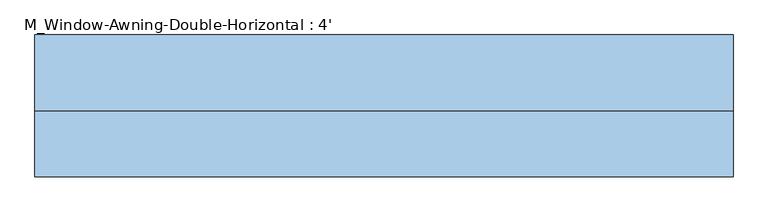
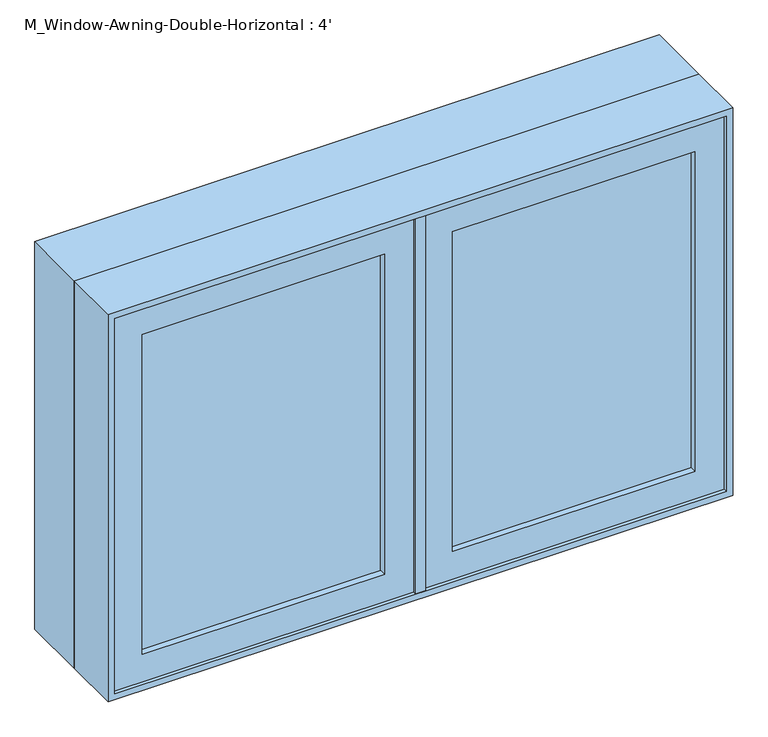
"""IFC4 building model written with IfcOpenShell, lengths in millimetres: window geometry, M_Window-Awning-Double-Horizontal : 4'."""

from ifc_helpers import new_model, si_unit, frame, origin, place, context, project, spatial, polyline, outline, extrude, faceted_brep, source, transform, mapped, element, save


def m_window_awning_double_horizontal_4_e2f7b2f6(model_context):
    return source(origin(), model_context, "Body", "SolidModel", [
        faceted_brep([(577.85, -82.55, 1668.25), (-577.85, -82.55, 1668.25), (-577.85, -19.05, 1668.25), (577.85, -19.05, 1668.25), (596.9, -133.35, 1687.3), (-596.9, -133.35, 1687.3), (-596.9, -82.55, 1687.3), (596.9, -82.55, 1687.3), (609.6, -19.05, 1700.0), (-609.6, -19.05, 1700.0), (-609.6, -133.35, 1700.0), (609.6, -133.35, 1700.0), (-577.85, -82.55, 931.75), (-577.85, -19.05, 931.75), (-596.9, -133.35, 912.7), (-596.9, -82.55, 912.7), (-609.6, -19.05, 900.0), (-609.6, -133.35, 900.0), (577.85, -82.55, 931.75), (577.85, -19.05, 931.75), (596.9, -133.35, 912.7), (596.9, -82.55, 912.7), (609.6, -19.05, 900.0), (609.6, -133.35, 900.0)], [[[0, 1, 2, 3]], [[4, 5, 6, 7]], [[8, 9, 10, 11]], [[1, 12, 13, 2]], [[5, 14, 15, 6]], [[9, 16, 17, 10]], [[12, 18, 19, 13]], [[14, 20, 21, 15]], [[16, 22, 23, 17]], [[9, 8, 22, 16], [3, 2, 13, 19]], [[18, 0, 3, 19]], [[7, 6, 15, 21], [1, 0, 18, 12]], [[20, 4, 7, 21]], [[22, 8, 11, 23]], [[11, 10, 17, 23], [5, 4, 20, 14]]]),
        extrude(outline(polyline([(1700.0, -609.6), (900.0, -609.6), (900.0, 609.6), (1700.0, 609.6), (1700.0, -609.6)]), holes=[polyline([(1680.95, 590.55), (919.05, 590.55), (919.05, -590.55), (1680.95, -590.55), (1680.95, 590.55)])]), frame((0.0, -19.05, 0.0), z_axis=(0.0, 1.0, 0.0), x_axis=(0.0, 0.0, 1.0)), (0.0, 0.0, 1.0), 133.35),
        extrude(outline(polyline([(912.7, 9.525), (912.7, 596.9), (1687.3, 596.9), (1687.3, 9.525), (912.7, 9.525)]), holes=[polyline([(969.85, 539.75), (969.85, 66.675), (1630.15, 66.675), (1630.15, 539.75), (969.85, 539.75)])]), frame((0.0, -127.0, 0.0), z_axis=(0.0, 1.0, 0.0), x_axis=(0.0, 0.0, 1.0)), (0.0, 0.0, 1.0), 44.45),
        extrude(outline(polyline([(1687.3, -9.525), (1687.3, -596.9), (912.7, -596.9), (912.7, -9.525), (1687.3, -9.525)]), holes=[polyline([(1630.15, -539.75), (1630.15, -66.675), (969.85, -66.675), (969.85, -539.75), (1630.15, -539.75)])]), frame((0.0, -127.0, 0.0), z_axis=(0.0, 1.0, 0.0), x_axis=(0.0, 0.0, 1.0)), (0.0, 0.0, 1.0), 44.45),
        extrude(outline(polyline([(539.75, -114.3), (66.675, -114.3), (66.675, -107.95), (539.75, -107.95), (539.75, -114.3)])), frame((0.0, 0.0, 969.85), z_axis=(0.0, 0.0, 1.0), x_axis=(1.0, 0.0, 0.0)), (0.0, 0.0, 1.0), 660.3),
        extrude(outline(polyline([(66.675, -95.25), (539.75, -95.25), (539.75, -101.6), (66.675, -101.6), (66.675, -95.25)])), frame((0.0, 0.0, 969.85), z_axis=(0.0, 0.0, 1.0), x_axis=(1.0, 0.0, 0.0)), (0.0, 0.0, 1.0), 660.3),
        extrude(outline(polyline([(-66.675, -114.3), (-539.75, -114.3), (-539.75, -107.95), (-66.675, -107.95), (-66.675, -114.3)])), frame((0.0, 0.0, 969.85), z_axis=(0.0, 0.0, 1.0), x_axis=(1.0, 0.0, 0.0)), (0.0, 0.0, 1.0), 660.3),
        extrude(outline(polyline([(-539.75, -95.25), (-66.675, -95.25), (-66.675, -101.6), (-539.75, -101.6), (-539.75, -95.25)])), frame((0.0, 0.0, 969.85), z_axis=(0.0, 0.0, 1.0), x_axis=(1.0, 0.0, 0.0)), (0.0, 0.0, 1.0), 660.3),
        faceted_brep([(9.525, -133.35, 1687.3), (9.525, -82.55, 1687.3), (-9.525, -82.55, 1687.3), (-9.525, -133.35, 1687.3), (9.525, -133.35, 912.7), (-9.525, -133.35, 912.7), (-9.525, -82.55, 912.7), (9.525, -82.55, 912.7), (-9.525, -82.55, 1668.25), (-9.525, -82.55, 931.75), (-30.1625, -82.55, 1668.25), (-30.1625, -82.55, 931.75), (-30.1625, -19.05, 1668.25), (-30.1625, -19.05, 931.75), (30.1625, -19.05, 1668.25), (30.1625, -19.05, 931.75), (30.1625, -82.55, 1668.25), (30.1625, -82.55, 931.75), (9.525, -82.55, 1668.25), (9.525, -82.55, 931.75)], [[[0, 1, 2, 3]], [[4, 5, 6, 7]], [[3, 5, 4, 0]], [[2, 8, 9, 6, 5, 3]], [[8, 10, 11, 9]], [[10, 12, 13, 11]], [[12, 14, 15, 13]], [[14, 16, 17, 15]], [[16, 18, 19, 17]], [[0, 4, 7, 19, 18, 1]], [[8, 2, 1, 18]], [[19, 7, 6, 9]], [[9, 11, 13, 15, 17, 19]], [[18, 16, 14, 12, 10, 8]]]),
    ])


if __name__ == "__main__":
    model = new_model("IFC4")
    model_context = context("Model", 3, world=origin())
    ifc_project = project(units=[si_unit("LENGTHUNIT", "METRE", prefix="MILLI")], contexts=[model_context])
    site = spatial("IfcSite", under=ifc_project)
    building = spatial("IfcBuilding", under=site)
    placement = place(None, origin())
    m_window_awning_double_horizontal_4_shape = m_window_awning_double_horizontal_4_e2f7b2f6(model_context)
    element("IfcWindow", 1, ObjectType="M_Window-Awning-Double-Horizontal : 4'", at=placement, inside=building, context=model_context, shape_type="MappedRepresentation", body=[
        mapped(m_window_awning_double_horizontal_4_shape, transform((0.0, 0.0, 0.0), x_axis=(1.0, 0.0, 0.0), y_axis=(0.0, 1.0, 0.0), z_axis=(0.0, 0.0, 1.0))),
    ])
    save(model, "model.ifc")

# Revit data of these elements
# Type "M_Window-Awning-Double-Horizontal : 4'"
#   Type Mark = "28"
#   Fire Rating = "0.5h"
#   Assembly Code = "B2020100"
#   Analytic Construction = "Double glazing - domestic"
#   Window Inset [instance default] = 0' - 0"
#   Wall Thickness [instance default] = 0' - 5.90551"
#   Interior Wall Closure [instance default] = 0' - 2.15551"
#   Half Width = 2' - 0"
#   Visual Light Transmittance = 0.81
#   Thermal Resistance (R) = 0.319569 (m²·K)/W
#   Solar Heat Gain Coefficient = 0.76
#   Rough Width = 4' - 0.59055"
#   Rough Height = 2' - 8.08661"
#   Height = 2' - 7.49606"
#   Heat Transfer Coefficient (U) = 3.12929 W/(m²·K)
#   Frame Extension [instance default] = 0' - 0 1/4"
#   Exterior Wall Closure [instance default] = 0' - 1 1/4"
#   Extension Jamb [instance default] = 0' - 2.15551"
#   Default Sill Height = 2' - 11.43307"
#   Width = 4' - 0"
#   Muntin Visibility = yes
#   Interior Trim Visibility [instance default] = yes
#   Exterior Trim Visibility [instance default] = yes
#   Extension Jamb Visibility [instance default] = yes
#   Interior Trim Material = Wood - Stained
#   Muntin Pattern = M_Muntin Pattern_2x2 : M_Muntin Pattern_2x2
#   Interior Trim = M_Trim-Window-Interior-Flat : Picture Frame
#   Interior Frame Material = Wood - Stained
#   Glass Panel Material = Glass
#   Exterior Trim Material = Clad - White
#   Exterior Trim = M_Trim-Window-Exterior-Flat : with Sill
#   Exterior Frame Material = Clad - White
#   Wall Closure = (empty or 0)
# Element 1 (IfcWindow, "M_Window-Awning-Double-Horizontal : 4'")
#   Wall Thickness = 0' - 9"
#   Extension Jamb = 0' - 5 1/4"
#   Materials on its faces: "Wood - Stained", "Glass", "Clad - White"
# Materials
#   "Wood - Stained": class "Wood", colour RGB 224 178 126, transparency 0, Cost = 0
#   "Glass": class "Glass", colour RGB 0 128 192, transparency 0.9, Description = "Soda Lime Glass", Cost = 0
#   "Clad - White": class "Wood", colour RGB 242 242 238, transparency 0, Cost = 0
